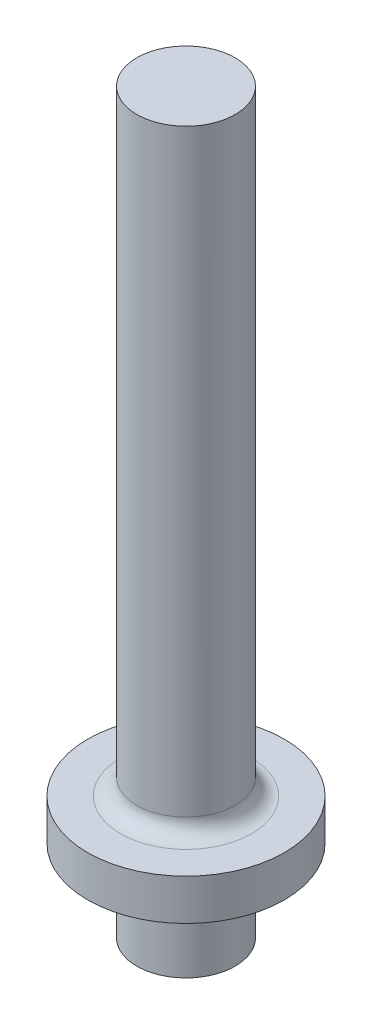
SolidWorks part; units mm, degrees
material "Plain Carbon Steel"
ref_plane "Front Plane" through (0, 0, 0) normal (0, 0, 1) x (1, 0, 0)
ref_plane "Top Plane" through (0, 0, 0) normal (0, 1, 0) x (1, 0, 0)
ref_plane "Right Plane" through (0, 0, 0) normal (1, 0, 0) x (0, 0, -1)
sketch "Stand Pin Profile" plane through (0, 0, 0) normal (0, 0, 1) x (1, 0, 0)
  line L0 (0, 0) -> (6, 0)
  line L1 (6, 0) -> (6, 10)
  line L2 (6, 15) -> (12, 15)
  line L3 (12, 15) -> (12, 10)
  line L4 (12, 10) -> (6, 10)
  line L5 (6, 15) -> (6, 90)
  line L6 (6, 90) -> (0, 90)
  line L7 (0, 90) -> (0, 0)
  dimension "D1" = 6
  dimension "D2" = 15
  dimension "D3" = 5
  dimension "D4" = 12
  dimension "D5" = 90
revolve "Stand Pin Body" add sketch "Stand Pin Profile" angle 360 about L7
fillet "Collar Fillet R2" radius 2 1 edges at (-6, 15, 0)
